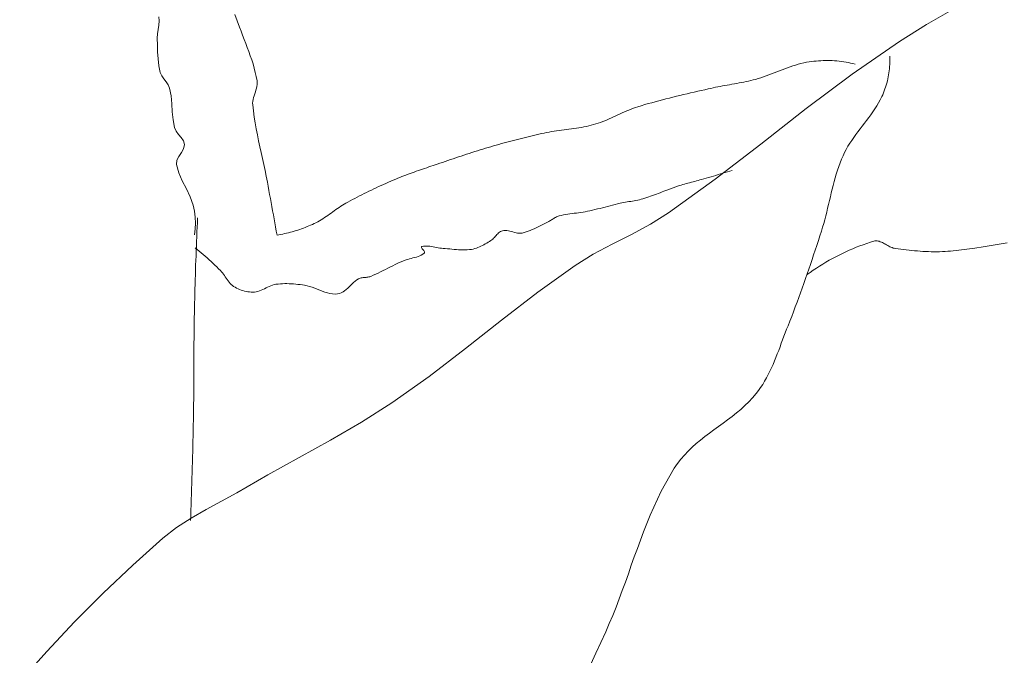
# Model space of a CAD drawing. Units: inches. Extents: x -36302355 to 648, y -221479757 to 75.
# Tile 33 of 37: x 284 to 311, y -20 to -2. Entities that reach past the tile are written whole.
import ezdxf

# ---------------------------------------------------------------- set-up
doc = ezdxf.new("R2010")
doc.units = ezdxf.units.IN
doc.header["$MEASUREMENT"] = 0
doc.layers.add('A-FURN', color=8, linetype='Continuous', lineweight=13)

# ---------------------------------------------------------------- blocks, each defined once
blk = doc.blocks.new('BED-DOUBLE')
for p, q in [((4.128, 63.666), (4.119, 63.783)), ((6.296, 63.67), (6.229, 63.842)), ((26.225, 64.013), (25.45, 63.569)), ((4.097, 63.43), (4.117, 63.548)), ((4.117, 63.548), (4.128, 63.666)), ((6.36, 63.496), (6.296, 63.67)), ((6.401, 63.383), (6.36, 63.496)), ((25.45, 63.569), (24.695, 63.097)), ((4.072, 63.192), (4.078, 63.311)), ((4.078, 63.311), (4.097, 63.43)), ((6.444, 63.269), (6.401, 63.383)), ((6.488, 63.156), (6.444, 63.269)), ((4.076, 62.999), (4.072, 63.192)), ((4.083, 62.806), (4.076, 62.999)), ((6.531, 63.043), (6.488, 63.156)), ((6.574, 62.929), (6.531, 63.043)), ((6.616, 62.816), (6.574, 62.929)), ((24.695, 63.097), (23.379, 62.192)), ((4.096, 62.613), (4.083, 62.806)), ((6.657, 62.702), (6.616, 62.816)), ((6.696, 62.587), (6.657, 62.702)), ((24.428, 62.63), (24.425, 62.688)), ((4.119, 62.421), (4.096, 62.613)), ((4.157, 62.233), (4.119, 62.421)), ((6.733, 62.472), (6.696, 62.587)), ((6.767, 62.356), (6.733, 62.472)), ((21.659, 62.392), (21.585, 62.366)), ((21.733, 62.418), (21.659, 62.392)), ((21.808, 62.442), (21.733, 62.418)), ((21.883, 62.464), (21.808, 62.442)), ((21.958, 62.485), (21.883, 62.464)), ((22.034, 62.503), (21.958, 62.485)), ((22.111, 62.519), (22.034, 62.503)), ((22.188, 62.532), (22.111, 62.519)), ((22.251, 62.541), (22.188, 62.532)), ((22.315, 62.549), (22.251, 62.541)), ((22.378, 62.555), (22.315, 62.549)), ((22.442, 62.561), (22.378, 62.555)), ((22.506, 62.564), (22.442, 62.561)), ((22.57, 62.567), (22.506, 62.564)), ((22.635, 62.568), (22.57, 62.567)), ((22.699, 62.568), (22.635, 62.568)), ((22.763, 62.567), (22.699, 62.568)), ((22.828, 62.565), (22.763, 62.567)), ((22.892, 62.561), (22.828, 62.565)), ((22.956, 62.556), (22.892, 62.561)), ((23.02, 62.55), (22.956, 62.556)), ((23.084, 62.542), (23.02, 62.55)), ((23.148, 62.533), (23.084, 62.542)), ((23.211, 62.523), (23.148, 62.533)), ((23.274, 62.512), (23.211, 62.523)), ((23.337, 62.499), (23.274, 62.512)), ((23.399, 62.485), (23.337, 62.499)), ((23.461, 62.47), (23.399, 62.485)), ((24.417, 62.342), (24.422, 62.4)), ((24.422, 62.4), (24.425, 62.458)), ((24.425, 62.458), (24.428, 62.515)), ((24.428, 62.573), (24.428, 62.63)), ((24.428, 62.515), (24.428, 62.573)), ((4.195, 62.142), (4.157, 62.233)), ((4.253, 62.059), (4.195, 62.142)), ((6.797, 62.24), (6.767, 62.356)), ((6.824, 62.122), (6.797, 62.24)), ((6.846, 62.004), (6.824, 62.122)), ((20.921, 62.115), (20.846, 62.09)), ((20.995, 62.141), (20.921, 62.115)), ((21.069, 62.168), (20.995, 62.141)), ((21.143, 62.196), (21.069, 62.168)), ((21.217, 62.224), (21.143, 62.196)), ((21.29, 62.253), (21.217, 62.224)), ((21.364, 62.282), (21.29, 62.253)), ((21.437, 62.31), (21.364, 62.282)), ((21.511, 62.338), (21.437, 62.31)), ((21.585, 62.366), (21.511, 62.338)), ((23.379, 62.192), (22.102, 61.232)), ((24.371, 62.056), (24.383, 62.113)), ((24.383, 62.113), (24.394, 62.17)), ((24.394, 62.17), (24.403, 62.227)), ((24.403, 62.227), (24.41, 62.285)), ((24.41, 62.285), (24.417, 62.342)), ((4.318, 61.979), (4.253, 62.059)), ((4.377, 61.896), (4.318, 61.979)), ((4.416, 61.805), (4.377, 61.896)), ((6.83, 61.798), (6.842, 61.849)), ((6.842, 61.849), (6.849, 61.9)), ((6.851, 61.952), (6.846, 62.004)), ((6.849, 61.9), (6.851, 61.952)), ((19.645, 61.837), (19.58, 61.824)), ((19.711, 61.849), (19.645, 61.837)), ((19.777, 61.862), (19.711, 61.849)), ((19.843, 61.873), (19.777, 61.862)), ((19.909, 61.885), (19.843, 61.873)), ((19.975, 61.897), (19.909, 61.885)), ((20.041, 61.909), (19.975, 61.897)), ((20.107, 61.92), (20.041, 61.909)), ((20.172, 61.932), (20.107, 61.92)), ((20.238, 61.945), (20.172, 61.932)), ((20.304, 61.957), (20.238, 61.945)), ((20.37, 61.97), (20.304, 61.957)), ((20.435, 61.984), (20.37, 61.97)), ((20.5, 61.998), (20.435, 61.984)), ((20.566, 62.013), (20.5, 61.998)), ((20.631, 62.029), (20.566, 62.013)), ((20.695, 62.046), (20.631, 62.029)), ((20.771, 62.067), (20.695, 62.046)), ((20.846, 62.09), (20.771, 62.067)), ((24.292, 61.778), (24.31, 61.833)), ((24.31, 61.833), (24.327, 61.888)), ((24.327, 61.888), (24.343, 61.944)), ((24.343, 61.944), (24.358, 62)), ((24.358, 62), (24.371, 62.056)), ((4.456, 61.588), (4.416, 61.805)), ((4.476, 61.367), (4.456, 61.588)), ((6.748, 61.541), (6.764, 61.592)), ((6.764, 61.592), (6.781, 61.644)), ((6.781, 61.644), (6.799, 61.695)), ((6.799, 61.695), (6.815, 61.746)), ((6.815, 61.746), (6.83, 61.798)), ((18.498, 61.574), (18.4, 61.551)), ((18.596, 61.598), (18.498, 61.574)), ((18.695, 61.621), (18.596, 61.598)), ((18.793, 61.645), (18.695, 61.621)), ((18.891, 61.667), (18.793, 61.645)), ((18.99, 61.69), (18.891, 61.667)), ((19.088, 61.713), (18.99, 61.69)), ((19.187, 61.736), (19.088, 61.713)), ((19.285, 61.759), (19.187, 61.736)), ((19.383, 61.781), (19.285, 61.759)), ((19.449, 61.796), (19.383, 61.781)), ((19.514, 61.81), (19.449, 61.796)), ((19.58, 61.824), (19.514, 61.81)), ((24.161, 61.478), (24.205, 61.565)), ((24.205, 61.565), (24.228, 61.618)), ((24.228, 61.618), (24.251, 61.67)), ((24.251, 61.67), (24.272, 61.724)), ((24.272, 61.724), (24.292, 61.778)), ((4.49, 61.145), (4.476, 61.367)), ((6.721, 61.386), (6.725, 61.438)), ((6.723, 61.334), (6.721, 61.386)), ((6.742, 61.167), (6.723, 61.334)), ((6.725, 61.438), (6.735, 61.489)), ((6.735, 61.489), (6.748, 61.541)), ((17.426, 61.284), (17.363, 61.264)), ((17.522, 61.314), (17.426, 61.284)), ((17.619, 61.343), (17.522, 61.314)), ((17.716, 61.371), (17.619, 61.343)), ((17.813, 61.398), (17.716, 61.371)), ((17.911, 61.425), (17.813, 61.398)), ((18.008, 61.451), (17.911, 61.425)), ((18.106, 61.477), (18.008, 61.451)), ((18.204, 61.502), (18.106, 61.477)), ((18.302, 61.526), (18.204, 61.502)), ((18.4, 61.551), (18.302, 61.526)), ((24.012, 61.225), (24.064, 61.308)), ((24.064, 61.308), (24.114, 61.392)), ((24.114, 61.392), (24.161, 61.478)), ((4.51, 60.924), (4.49, 61.145)), ((6.765, 61), (6.742, 61.167)), ((16.813, 61.032), (16.752, 61.004)), ((16.873, 61.06), (16.813, 61.032)), ((16.934, 61.087), (16.873, 61.06)), ((16.994, 61.115), (16.934, 61.087)), ((17.055, 61.142), (16.994, 61.115)), ((17.116, 61.168), (17.055, 61.142)), ((17.177, 61.194), (17.116, 61.168)), ((17.238, 61.218), (17.177, 61.194)), ((17.3, 61.242), (17.238, 61.218)), ((17.363, 61.264), (17.3, 61.242)), ((22.102, 61.232), (20.841, 60.248)), ((23.842, 60.984), (23.9, 61.063)), ((23.9, 61.063), (23.957, 61.144)), ((23.957, 61.144), (24.012, 61.225)), ((4.551, 60.707), (4.51, 60.924)), ((6.792, 60.835), (6.765, 61)), ((6.821, 60.669), (6.792, 60.835)), ((15.994, 60.739), (15.926, 60.726)), ((16.062, 60.754), (15.994, 60.739)), ((16.13, 60.771), (16.062, 60.754)), ((16.197, 60.789), (16.13, 60.771)), ((16.261, 60.808), (16.197, 60.789)), ((16.323, 60.828), (16.261, 60.808)), ((16.386, 60.85), (16.323, 60.828)), ((16.448, 60.874), (16.386, 60.85)), ((16.509, 60.898), (16.448, 60.874)), ((16.57, 60.924), (16.509, 60.898)), ((16.631, 60.95), (16.57, 60.924)), ((16.692, 60.977), (16.631, 60.95)), ((16.752, 61.004), (16.692, 60.977)), ((23.602, 60.669), (23.662, 60.748)), ((23.662, 60.748), (23.723, 60.826)), ((23.723, 60.826), (23.783, 60.905)), ((23.783, 60.905), (23.842, 60.984)), ((4.596, 60.607), (4.551, 60.707)), ((4.665, 60.516), (4.596, 60.607)), ((4.738, 60.428), (4.665, 60.516)), ((6.853, 60.504), (6.821, 60.669)), ((6.887, 60.34), (6.853, 60.504)), ((14.45, 60.47), (14.376, 60.452)), ((14.524, 60.487), (14.45, 60.47)), ((14.599, 60.504), (14.524, 60.487)), ((14.673, 60.521), (14.599, 60.504)), ((14.748, 60.538), (14.673, 60.521)), ((14.822, 60.554), (14.748, 60.538)), ((14.891, 60.568), (14.822, 60.554)), ((14.959, 60.581), (14.891, 60.568)), ((15.028, 60.593), (14.959, 60.581)), ((15.097, 60.604), (15.028, 60.593)), ((15.166, 60.614), (15.097, 60.604)), ((15.235, 60.624), (15.166, 60.614)), ((15.304, 60.633), (15.235, 60.624)), ((15.374, 60.642), (15.304, 60.633)), ((15.443, 60.652), (15.374, 60.642)), ((15.512, 60.661), (15.443, 60.652)), ((15.582, 60.67), (15.512, 60.661)), ((15.651, 60.68), (15.582, 60.67)), ((15.72, 60.69), (15.651, 60.68)), ((15.789, 60.701), (15.72, 60.69)), ((15.857, 60.713), (15.789, 60.701)), ((15.926, 60.726), (15.857, 60.713)), ((23.426, 60.431), (23.484, 60.511)), ((23.484, 60.511), (23.542, 60.59)), ((23.542, 60.59), (23.602, 60.669)), ((4.798, 60.335), (4.738, 60.428)), ((4.826, 60.233), (4.798, 60.335)), ((4.805, 60.119), (4.826, 60.233)), ((6.922, 60.175), (6.887, 60.34)), ((13.416, 60.198), (13.343, 60.176)), ((13.489, 60.219), (13.416, 60.198)), ((13.563, 60.239), (13.489, 60.219)), ((13.636, 60.26), (13.563, 60.239)), ((13.71, 60.28), (13.636, 60.26)), ((13.784, 60.3), (13.71, 60.28)), ((13.857, 60.32), (13.784, 60.3)), ((13.931, 60.34), (13.857, 60.32)), ((14.005, 60.359), (13.931, 60.34)), ((14.079, 60.378), (14.005, 60.359)), ((14.153, 60.397), (14.079, 60.378)), ((14.227, 60.416), (14.153, 60.397)), ((14.301, 60.434), (14.227, 60.416)), ((14.376, 60.452), (14.301, 60.434)), ((20.841, 60.248), (19.575, 59.272)), ((23.264, 60.186), (23.316, 60.269)), ((23.316, 60.269), (23.37, 60.351)), ((23.37, 60.351), (23.426, 60.431)), ((4.675, 59.905), (4.746, 60.011)), ((4.746, 60.011), (4.805, 60.119)), ((6.958, 60.011), (6.922, 60.175)), ((6.994, 59.846), (6.958, 60.011)), ((12.519, 59.917), (12.445, 59.892)), ((12.594, 59.942), (12.519, 59.917)), ((12.668, 59.967), (12.594, 59.942)), ((12.743, 59.991), (12.668, 59.967)), ((12.817, 60.015), (12.743, 59.991)), ((12.892, 60.039), (12.817, 60.015)), ((12.967, 60.063), (12.892, 60.039)), ((13.042, 60.086), (12.967, 60.063)), ((13.117, 60.109), (13.042, 60.086)), ((13.192, 60.132), (13.117, 60.109)), ((13.267, 60.154), (13.192, 60.132)), ((13.343, 60.176), (13.267, 60.154)), ((23.085, 59.826), (23.128, 59.926)), ((23.128, 59.926), (23.17, 60.015)), ((23.17, 60.015), (23.215, 60.101)), ((23.215, 60.101), (23.264, 60.186)), ((4.607, 59.685), (4.62, 59.798)), ((4.668, 59.449), (4.607, 59.685)), ((4.62, 59.798), (4.675, 59.905)), ((7.03, 59.682), (6.994, 59.846)), ((7.066, 59.517), (7.03, 59.682)), ((11.734, 59.651), (11.676, 59.631)), ((11.792, 59.671), (11.734, 59.651)), ((11.85, 59.69), (11.792, 59.671)), ((11.924, 59.716), (11.85, 59.69)), ((11.999, 59.741), (11.924, 59.716)), ((12.073, 59.766), (11.999, 59.741)), ((12.147, 59.792), (12.073, 59.766)), ((12.221, 59.817), (12.147, 59.792)), ((12.296, 59.842), (12.221, 59.817)), ((12.37, 59.867), (12.296, 59.842)), ((12.445, 59.892), (12.37, 59.867)), ((23.007, 59.623), (23.045, 59.725)), ((23.045, 59.725), (23.085, 59.826)), ((4.766, 59.224), (4.668, 59.449)), ((7.1, 59.353), (7.066, 59.517)), ((10.924, 59.366), (10.867, 59.344)), ((10.981, 59.388), (10.924, 59.366)), ((11.039, 59.41), (10.981, 59.388)), ((11.096, 59.431), (11.039, 59.41)), ((11.154, 59.452), (11.096, 59.431)), ((11.212, 59.472), (11.154, 59.452)), ((11.269, 59.493), (11.212, 59.472)), ((11.327, 59.513), (11.269, 59.493)), ((11.385, 59.533), (11.327, 59.513)), ((11.443, 59.553), (11.385, 59.533)), ((11.501, 59.572), (11.443, 59.553)), ((11.56, 59.592), (11.501, 59.572)), ((11.618, 59.612), (11.56, 59.592)), ((11.676, 59.631), (11.618, 59.612)), ((19.588, 59.379), (19.523, 59.36)), ((19.653, 59.399), (19.588, 59.379)), ((19.718, 59.418), (19.653, 59.399)), ((19.783, 59.438), (19.718, 59.418)), ((19.848, 59.458), (19.783, 59.438)), ((19.913, 59.478), (19.848, 59.458)), ((19.978, 59.498), (19.913, 59.478)), ((20.043, 59.518), (19.978, 59.498)), ((22.909, 59.313), (22.94, 59.417)), ((22.94, 59.417), (22.973, 59.521)), ((22.973, 59.521), (23.007, 59.623)), ((4.88, 59.003), (4.766, 59.224)), ((7.132, 59.188), (7.1, 59.353)), ((7.153, 59.075), (7.132, 59.188)), ((10.29, 59.097), (10.223, 59.066)), ((10.358, 59.127), (10.29, 59.097)), ((10.425, 59.157), (10.358, 59.127)), ((10.493, 59.187), (10.425, 59.157)), ((10.561, 59.216), (10.493, 59.187)), ((10.629, 59.246), (10.561, 59.216)), ((10.697, 59.275), (10.629, 59.246)), ((10.753, 59.298), (10.697, 59.275)), ((10.81, 59.321), (10.753, 59.298)), ((10.867, 59.344), (10.81, 59.321)), ((19.575, 59.272), (18.281, 58.335)), ((18.58, 59.094), (18.555, 59.086)), ((18.627, 59.108), (18.58, 59.094)), ((18.675, 59.122), (18.627, 59.108)), ((18.722, 59.135), (18.675, 59.122)), ((18.769, 59.149), (18.722, 59.135)), ((18.817, 59.161), (18.769, 59.149)), ((18.864, 59.174), (18.817, 59.161)), ((18.912, 59.187), (18.864, 59.174)), ((18.959, 59.199), (18.912, 59.187)), ((19.007, 59.212), (18.959, 59.199)), ((19.054, 59.225), (19.007, 59.212)), ((19.102, 59.238), (19.054, 59.225)), ((19.149, 59.251), (19.102, 59.238)), ((19.197, 59.264), (19.149, 59.251)), ((19.262, 59.283), (19.197, 59.264)), ((19.327, 59.302), (19.262, 59.283)), ((19.392, 59.321), (19.327, 59.302)), ((19.458, 59.341), (19.392, 59.321)), ((19.523, 59.36), (19.458, 59.341)), ((22.826, 58.996), (22.852, 59.102)), ((22.852, 59.102), (22.88, 59.208)), ((22.88, 59.208), (22.909, 59.313)), ((4.988, 58.78), (4.88, 59.003)), ((7.174, 58.962), (7.153, 59.075)), ((7.195, 58.849), (7.174, 58.962)), ((7.216, 58.737), (7.195, 58.849)), ((9.756, 58.842), (9.69, 58.809)), ((9.822, 58.875), (9.756, 58.842)), ((9.889, 58.908), (9.822, 58.875)), ((9.955, 58.94), (9.889, 58.908)), ((10.022, 58.972), (9.955, 58.94)), ((10.089, 59.004), (10.022, 58.972)), ((10.156, 59.035), (10.089, 59.004)), ((10.223, 59.066), (10.156, 59.035)), ((17.887, 58.837), (17.834, 58.817)), ((17.94, 58.857), (17.887, 58.837)), ((17.993, 58.877), (17.94, 58.857)), ((18.046, 58.898), (17.993, 58.877)), ((18.098, 58.918), (18.046, 58.898)), ((18.151, 58.938), (18.098, 58.918)), ((18.204, 58.958), (18.151, 58.938)), ((18.257, 58.978), (18.204, 58.958)), ((18.282, 58.987), (18.257, 58.978)), ((18.307, 58.996), (18.282, 58.987)), ((18.332, 59.005), (18.307, 58.996)), ((18.356, 59.015), (18.332, 59.005)), ((18.381, 59.024), (18.356, 59.015)), ((18.406, 59.033), (18.381, 59.024)), ((18.431, 59.043), (18.406, 59.033)), ((18.455, 59.052), (18.431, 59.043)), ((18.48, 59.061), (18.455, 59.052)), ((18.505, 59.07), (18.48, 59.061)), ((18.53, 59.078), (18.505, 59.07)), ((18.555, 59.086), (18.53, 59.078)), ((22.775, 58.784), (22.8, 58.89)), ((22.8, 58.89), (22.826, 58.996)), ((5.069, 58.548), (4.988, 58.78)), ((5.103, 58.387), (5.069, 58.548)), ((7.236, 58.624), (7.216, 58.737)), ((7.257, 58.511), (7.236, 58.624)), ((9.22, 58.553), (9.174, 58.522)), ((9.267, 58.582), (9.22, 58.553)), ((9.315, 58.61), (9.267, 58.582)), ((9.363, 58.637), (9.315, 58.61)), ((9.428, 58.672), (9.363, 58.637)), ((9.493, 58.707), (9.428, 58.672)), ((9.559, 58.741), (9.493, 58.707)), ((9.624, 58.776), (9.559, 58.741)), ((9.69, 58.809), (9.624, 58.776)), ((16.723, 58.554), (16.653, 58.536)), ((16.792, 58.571), (16.723, 58.554)), ((16.862, 58.588), (16.792, 58.571)), ((16.933, 58.604), (16.862, 58.588)), ((16.981, 58.615), (16.933, 58.604)), ((17.03, 58.624), (16.981, 58.615)), ((17.079, 58.633), (17.03, 58.624)), ((17.128, 58.642), (17.079, 58.633)), ((17.177, 58.65), (17.128, 58.642)), ((17.226, 58.658), (17.177, 58.65)), ((17.275, 58.666), (17.226, 58.658)), ((17.324, 58.675), (17.275, 58.666)), ((17.372, 58.684), (17.324, 58.675)), ((17.421, 58.693), (17.372, 58.684)), ((17.469, 58.704), (17.421, 58.693)), ((17.518, 58.716), (17.469, 58.704)), ((17.566, 58.728), (17.518, 58.716)), ((17.62, 58.744), (17.566, 58.728)), ((17.674, 58.761), (17.62, 58.744)), ((17.727, 58.779), (17.674, 58.761)), ((17.781, 58.798), (17.727, 58.779)), ((17.834, 58.817), (17.781, 58.798)), ((22.699, 58.465), (22.725, 58.571)), ((22.725, 58.571), (22.75, 58.678)), ((22.75, 58.678), (22.775, 58.784)), ((5.123, 58.222), (5.103, 58.387)), ((7.278, 58.398), (7.257, 58.511)), ((7.298, 58.285), (7.278, 58.398)), ((7.319, 58.172), (7.298, 58.285)), ((8.856, 58.299), (8.81, 58.267)), ((8.901, 58.331), (8.856, 58.299)), ((8.946, 58.364), (8.901, 58.331)), ((8.991, 58.396), (8.946, 58.364)), ((9.037, 58.428), (8.991, 58.396)), ((9.082, 58.46), (9.037, 58.428)), ((9.128, 58.491), (9.082, 58.46)), ((9.174, 58.522), (9.128, 58.491)), ((15.355, 58.28), (15.295, 58.267)), ((15.415, 58.291), (15.355, 58.28)), ((15.476, 58.301), (15.415, 58.291)), ((15.536, 58.31), (15.476, 58.301)), ((15.597, 58.318), (15.536, 58.31)), ((15.658, 58.326), (15.597, 58.318)), ((15.719, 58.333), (15.658, 58.326)), ((15.78, 58.341), (15.719, 58.333)), ((15.841, 58.35), (15.78, 58.341)), ((15.902, 58.359), (15.841, 58.35)), ((15.963, 58.369), (15.902, 58.359)), ((16.023, 58.381), (15.963, 58.369)), ((16.093, 58.396), (16.023, 58.381)), ((16.164, 58.412), (16.093, 58.396)), ((16.234, 58.428), (16.164, 58.412)), ((16.304, 58.446), (16.234, 58.428)), ((16.374, 58.463), (16.304, 58.446)), ((16.443, 58.481), (16.374, 58.463)), ((16.513, 58.5), (16.443, 58.481)), ((16.583, 58.518), (16.513, 58.5)), ((16.653, 58.536), (16.583, 58.518)), ((18.281, 58.335), (17.775, 58.02)), ((22.647, 58.252), (22.674, 58.358)), ((22.674, 58.358), (22.699, 58.465)), ((5.13, 58.056), (5.123, 58.222)), ((5.124, 57.891), (5.13, 58.056)), ((5.181, 57.938), (5.187, 58.07)), ((5.187, 58.07), (5.194, 58.202)), ((7.339, 58.06), (7.319, 58.172)), ((7.36, 57.947), (7.339, 58.06)), ((8.382, 58.018), (8.333, 57.996)), ((8.431, 58.041), (8.382, 58.018)), ((8.481, 58.065), (8.431, 58.041)), ((8.53, 58.09), (8.481, 58.065)), ((8.578, 58.117), (8.53, 58.09)), ((8.626, 58.146), (8.578, 58.117)), ((8.672, 58.175), (8.626, 58.146)), ((8.719, 58.205), (8.672, 58.175)), ((8.765, 58.236), (8.719, 58.205)), ((8.81, 58.267), (8.765, 58.236)), ((14.766, 58.009), (14.711, 57.981)), ((14.82, 58.037), (14.766, 58.009)), ((14.874, 58.064), (14.82, 58.037)), ((14.929, 58.09), (14.874, 58.064)), ((14.953, 58.102), (14.929, 58.09)), ((14.976, 58.115), (14.953, 58.102)), ((15, 58.128), (14.976, 58.115)), ((15.022, 58.143), (15, 58.128)), ((15.045, 58.157), (15.022, 58.143)), ((15.068, 58.171), (15.045, 58.157)), ((15.091, 58.186), (15.068, 58.171)), ((15.114, 58.199), (15.091, 58.186)), ((15.137, 58.213), (15.114, 58.199)), ((15.161, 58.225), (15.137, 58.213)), ((15.185, 58.236), (15.161, 58.225)), ((15.21, 58.245), (15.185, 58.236)), ((15.235, 58.253), (15.21, 58.245)), ((15.295, 58.267), (15.235, 58.253)), ((17.775, 58.02), (17.248, 57.739)), ((22.56, 57.937), (22.59, 58.042)), ((22.59, 58.042), (22.619, 58.147)), ((22.619, 58.147), (22.647, 58.252)), ((5.104, 57.727), (5.124, 57.891)), ((5.17, 57.675), (5.176, 57.807)), ((5.176, 57.807), (5.181, 57.938)), ((7.38, 57.834), (7.36, 57.947)), ((7.4, 57.721), (7.38, 57.834)), ((7.453, 57.73), (7.4, 57.721)), ((7.506, 57.74), (7.453, 57.73)), ((7.559, 57.751), (7.506, 57.74)), ((7.612, 57.762), (7.559, 57.751)), ((7.665, 57.774), (7.612, 57.762)), ((7.718, 57.787), (7.665, 57.774)), ((7.77, 57.801), (7.718, 57.787)), ((7.823, 57.815), (7.77, 57.801)), ((7.875, 57.83), (7.823, 57.815)), ((7.927, 57.846), (7.875, 57.83)), ((7.978, 57.862), (7.927, 57.846)), ((8.03, 57.879), (7.978, 57.862)), ((8.081, 57.897), (8.03, 57.879)), ((8.132, 57.916), (8.081, 57.897)), ((8.183, 57.935), (8.132, 57.916)), ((8.233, 57.955), (8.183, 57.935)), ((8.283, 57.975), (8.233, 57.955)), ((8.333, 57.996), (8.283, 57.975)), ((13.509, 57.734), (13.486, 57.709)), ((13.531, 57.758), (13.509, 57.734)), ((13.554, 57.781), (13.531, 57.758)), ((13.579, 57.801), (13.554, 57.781)), ((13.605, 57.819), (13.579, 57.801)), ((13.633, 57.832), (13.605, 57.819)), ((13.663, 57.842), (13.633, 57.832)), ((13.704, 57.849), (13.663, 57.842)), ((13.746, 57.85), (13.704, 57.849)), ((13.787, 57.847), (13.746, 57.85)), ((13.829, 57.84), (13.787, 57.847)), ((13.871, 57.83), (13.829, 57.84)), ((13.914, 57.819), (13.871, 57.83)), ((13.956, 57.807), (13.914, 57.819)), ((13.998, 57.795), (13.956, 57.807)), ((14.04, 57.785), (13.998, 57.795)), ((14.082, 57.778), (14.04, 57.785)), ((14.124, 57.773), (14.082, 57.778)), ((14.166, 57.773), (14.124, 57.773)), ((14.208, 57.778), (14.166, 57.773)), ((14.266, 57.791), (14.208, 57.778)), ((14.324, 57.808), (14.266, 57.791)), ((14.381, 57.827), (14.324, 57.808)), ((14.437, 57.849), (14.381, 57.827)), ((14.493, 57.873), (14.437, 57.849)), ((14.548, 57.899), (14.493, 57.873)), ((14.603, 57.925), (14.548, 57.899)), ((14.657, 57.953), (14.603, 57.925)), ((14.711, 57.981), (14.657, 57.953)), ((17.248, 57.739), (16.714, 57.469)), ((22.484, 57.701), (22.527, 57.833)), ((22.527, 57.833), (22.56, 57.937)), ((5.159, 57.411), (5.164, 57.543)), ((5.164, 57.543), (5.17, 57.675)), ((13.146, 57.454), (13.106, 57.432)), ((13.186, 57.477), (13.146, 57.454)), ((13.226, 57.5), (13.186, 57.477)), ((13.266, 57.523), (13.226, 57.5)), ((13.305, 57.547), (13.266, 57.523)), ((13.344, 57.571), (13.305, 57.547)), ((13.371, 57.589), (13.344, 57.571)), ((13.396, 57.61), (13.371, 57.589)), ((13.419, 57.633), (13.396, 57.61)), ((13.442, 57.658), (13.419, 57.633)), ((13.464, 57.683), (13.442, 57.658)), ((13.486, 57.709), (13.464, 57.683)), ((16.714, 57.469), (16.186, 57.189)), ((22.398, 57.436), (22.441, 57.568)), ((22.441, 57.568), (22.484, 57.701)), ((23.688, 57.454), (23.59, 57.418)), ((23.786, 57.488), (23.688, 57.454)), ((23.885, 57.52), (23.786, 57.488)), ((23.984, 57.551), (23.885, 57.52)), ((24.014, 57.558), (23.984, 57.551)), ((24.044, 57.56), (24.014, 57.558)), ((24.074, 57.559), (24.044, 57.56)), ((24.103, 57.555), (24.074, 57.559)), ((24.133, 57.548), (24.103, 57.555)), ((24.162, 57.538), (24.133, 57.548)), ((24.191, 57.526), (24.162, 57.538)), ((24.22, 57.513), (24.191, 57.526)), ((24.25, 57.498), (24.22, 57.513)), ((24.279, 57.482), (24.25, 57.498)), ((24.308, 57.465), (24.279, 57.482)), ((24.338, 57.448), (24.308, 57.465)), ((27.467, 57.465), (27.243, 57.428)), ((27.691, 57.503), (27.467, 57.465)), ((5.185, 57.325), (5.129, 57.371)), ((5.149, 57.147), (5.154, 57.279)), ((5.154, 57.279), (5.159, 57.411)), ((5.24, 57.278), (5.185, 57.325)), ((5.295, 57.231), (5.24, 57.278)), ((5.35, 57.183), (5.295, 57.231)), ((5.405, 57.135), (5.35, 57.183)), ((11.451, 57.188), (11.409, 57.165)), ((11.414, 57.394), (11.411, 57.385)), ((11.411, 57.385), (11.414, 57.373)), ((11.425, 57.4), (11.414, 57.394)), ((11.414, 57.373), (11.422, 57.359)), ((11.422, 57.359), (11.433, 57.343)), ((11.469, 57.409), (11.425, 57.4)), ((11.433, 57.343), (11.447, 57.325)), ((11.447, 57.325), (11.461, 57.307)), ((11.491, 57.216), (11.451, 57.188)), ((11.461, 57.307), (11.475, 57.289)), ((11.514, 57.414), (11.469, 57.409)), ((11.475, 57.289), (11.487, 57.271)), ((11.487, 57.271), (11.496, 57.255)), ((11.5, 57.226), (11.491, 57.216)), ((11.496, 57.255), (11.501, 57.239)), ((11.501, 57.239), (11.5, 57.226)), ((11.559, 57.415), (11.514, 57.414)), ((11.604, 57.413), (11.559, 57.415)), ((11.649, 57.409), (11.604, 57.413)), ((11.695, 57.403), (11.649, 57.409)), ((11.741, 57.395), (11.695, 57.403)), ((11.787, 57.386), (11.741, 57.395)), ((11.832, 57.378), (11.787, 57.386)), ((11.878, 57.369), (11.832, 57.378)), ((11.924, 57.362), (11.878, 57.369)), ((11.97, 57.356), (11.924, 57.362)), ((12.015, 57.352), (11.97, 57.356)), ((12.076, 57.348), (12.015, 57.352)), ((12.137, 57.343), (12.076, 57.348)), ((12.198, 57.338), (12.137, 57.343)), ((12.26, 57.331), (12.198, 57.338)), ((12.321, 57.325), (12.26, 57.331)), ((12.382, 57.32), (12.321, 57.325)), ((12.443, 57.315), (12.382, 57.32)), ((12.504, 57.311), (12.443, 57.315)), ((12.565, 57.309), (12.504, 57.311)), ((12.626, 57.309), (12.565, 57.309)), ((12.686, 57.312), (12.626, 57.309)), ((12.747, 57.317), (12.686, 57.312)), ((12.807, 57.325), (12.747, 57.317)), ((12.852, 57.334), (12.807, 57.325)), ((12.895, 57.345), (12.852, 57.334)), ((12.939, 57.359), (12.895, 57.345)), ((12.981, 57.375), (12.939, 57.359)), ((13.023, 57.392), (12.981, 57.375)), ((13.065, 57.412), (13.023, 57.392)), ((13.106, 57.432), (13.065, 57.412)), ((16.186, 57.189), (15.68, 56.875)), ((22.31, 57.171), (22.354, 57.303)), ((22.354, 57.303), (22.398, 57.436)), ((23.11, 57.213), (23.017, 57.167)), ((23.205, 57.258), (23.11, 57.213)), ((23.3, 57.3), (23.205, 57.258)), ((23.396, 57.341), (23.3, 57.3)), ((23.493, 57.381), (23.396, 57.341)), ((23.59, 57.418), (23.493, 57.381)), ((24.367, 57.431), (24.338, 57.448)), ((24.397, 57.415), (24.367, 57.431)), ((24.426, 57.399), (24.397, 57.415)), ((24.456, 57.385), (24.426, 57.399)), ((24.487, 57.372), (24.456, 57.385)), ((24.517, 57.362), (24.487, 57.372)), ((24.548, 57.354), (24.517, 57.362)), ((24.579, 57.348), (24.548, 57.354)), ((24.655, 57.338), (24.579, 57.348)), ((24.732, 57.329), (24.655, 57.338)), ((24.808, 57.32), (24.732, 57.329)), ((24.885, 57.311), (24.808, 57.32)), ((24.962, 57.302), (24.885, 57.311)), ((25.039, 57.294), (24.962, 57.302)), ((25.116, 57.287), (25.039, 57.294)), ((25.193, 57.28), (25.116, 57.287)), ((25.27, 57.274), (25.193, 57.28)), ((25.347, 57.269), (25.27, 57.274)), ((25.424, 57.264), (25.347, 57.269)), ((25.501, 57.261), (25.424, 57.264)), ((25.578, 57.258), (25.501, 57.261)), ((25.655, 57.257), (25.578, 57.258)), ((25.732, 57.257), (25.655, 57.257)), ((25.809, 57.258), (25.732, 57.257)), ((25.886, 57.261), (25.809, 57.258)), ((25.963, 57.265), (25.886, 57.261)), ((26.039, 57.27), (25.963, 57.265)), ((26.116, 57.277), (26.039, 57.27)), ((26.342, 57.302), (26.116, 57.277)), ((26.568, 57.329), (26.342, 57.302)), ((26.793, 57.36), (26.568, 57.329)), ((27.018, 57.393), (26.793, 57.36)), ((27.243, 57.428), (27.018, 57.393)), ((5.139, 56.883), (5.144, 57.015)), ((5.144, 57.015), (5.149, 57.147)), ((5.459, 57.087), (5.405, 57.135)), ((5.513, 57.038), (5.459, 57.087)), ((5.566, 56.989), (5.513, 57.038)), ((5.619, 56.939), (5.566, 56.989)), ((5.671, 56.889), (5.619, 56.939)), ((10.754, 56.937), (10.685, 56.904)), ((10.822, 56.969), (10.754, 56.937)), ((10.892, 56.999), (10.822, 56.969)), ((10.937, 57.017), (10.892, 56.999)), ((10.984, 57.033), (10.937, 57.017)), ((11.032, 57.047), (10.984, 57.033)), ((11.08, 57.06), (11.032, 57.047)), ((11.129, 57.073), (11.08, 57.06)), ((11.177, 57.085), (11.129, 57.073)), ((11.225, 57.098), (11.177, 57.085)), ((11.273, 57.111), (11.225, 57.098)), ((11.319, 57.127), (11.273, 57.111)), ((11.365, 57.144), (11.319, 57.127)), ((11.409, 57.165), (11.365, 57.144)), ((22.177, 56.774), (22.221, 56.906)), ((22.221, 56.906), (22.266, 57.039)), ((22.266, 57.039), (22.31, 57.171)), ((22.561, 56.913), (22.472, 56.858)), ((22.65, 56.967), (22.561, 56.913)), ((22.74, 57.02), (22.65, 56.967)), ((22.831, 57.07), (22.74, 57.02)), ((22.924, 57.12), (22.831, 57.07)), ((23.017, 57.167), (22.924, 57.12)), ((5.131, 56.619), (5.135, 56.751)), ((5.135, 56.751), (5.139, 56.883)), ((5.723, 56.839), (5.671, 56.889)), ((5.775, 56.788), (5.723, 56.839)), ((5.826, 56.736), (5.775, 56.788)), ((5.856, 56.704), (5.826, 56.736)), ((5.885, 56.67), (5.856, 56.704)), ((5.911, 56.634), (5.885, 56.67)), ((5.937, 56.597), (5.911, 56.634)), ((10.142, 56.634), (10.073, 56.604)), ((10.211, 56.666), (10.142, 56.634)), ((10.279, 56.699), (10.211, 56.666)), ((10.347, 56.733), (10.279, 56.699)), ((10.414, 56.767), (10.347, 56.733)), ((10.482, 56.801), (10.414, 56.767)), ((10.55, 56.836), (10.482, 56.801)), ((10.617, 56.87), (10.55, 56.836)), ((10.685, 56.904), (10.617, 56.87)), ((15.68, 56.875), (14.648, 56.132)), ((22.086, 56.511), (22.131, 56.643)), ((22.214, 56.683), (22.13, 56.622)), ((22.131, 56.643), (22.177, 56.774)), ((22.299, 56.743), (22.214, 56.683)), ((22.385, 56.801), (22.299, 56.743)), ((22.472, 56.858), (22.385, 56.801)), ((5.123, 56.355), (5.127, 56.487)), ((5.127, 56.487), (5.131, 56.619)), ((5.962, 56.559), (5.937, 56.597)), ((5.987, 56.522), (5.962, 56.559)), ((6.013, 56.485), (5.987, 56.522)), ((6.039, 56.449), (6.013, 56.485)), ((6.066, 56.414), (6.039, 56.449)), ((6.095, 56.38), (6.066, 56.414)), ((6.125, 56.349), (6.095, 56.38)), ((7.432, 56.362), (7.371, 56.355)), ((7.492, 56.368), (7.432, 56.362)), ((7.553, 56.371), (7.492, 56.368)), ((7.614, 56.373), (7.553, 56.371)), ((7.676, 56.373), (7.614, 56.373)), ((7.737, 56.371), (7.676, 56.373)), ((7.798, 56.369), (7.737, 56.371)), ((7.859, 56.365), (7.798, 56.369)), ((7.92, 56.359), (7.859, 56.365)), ((7.981, 56.353), (7.92, 56.359)), ((9.486, 56.366), (9.445, 56.325)), ((9.528, 56.405), (9.486, 56.366)), ((9.571, 56.442), (9.528, 56.405)), ((9.616, 56.476), (9.571, 56.442)), ((9.663, 56.504), (9.616, 56.476)), ((9.687, 56.515), (9.663, 56.504)), ((9.712, 56.524), (9.687, 56.515)), ((9.738, 56.53), (9.712, 56.524)), ((9.764, 56.535), (9.738, 56.53)), ((9.79, 56.539), (9.764, 56.535)), ((9.817, 56.542), (9.79, 56.539)), ((9.844, 56.545), (9.817, 56.542)), ((9.872, 56.547), (9.844, 56.545)), ((9.899, 56.55), (9.872, 56.547)), ((9.925, 56.554), (9.899, 56.55)), ((9.952, 56.559), (9.925, 56.554)), ((9.977, 56.566), (9.952, 56.559)), ((10.003, 56.574), (9.977, 56.566)), ((10.073, 56.604), (10.003, 56.574)), ((21.993, 56.248), (22.039, 56.379)), ((22.039, 56.379), (22.086, 56.511)), ((5.112, 55.959), (5.115, 56.091)), ((5.115, 56.091), (5.119, 56.223)), ((5.119, 56.223), (5.123, 56.355)), ((6.158, 56.321), (6.125, 56.349)), ((6.194, 56.296), (6.158, 56.321)), ((6.234, 56.272), (6.194, 56.296)), ((6.274, 56.25), (6.234, 56.272)), ((6.317, 56.229), (6.274, 56.25)), ((6.36, 56.211), (6.317, 56.229)), ((6.404, 56.195), (6.36, 56.211)), ((6.449, 56.18), (6.404, 56.195)), ((6.494, 56.168), (6.449, 56.18)), ((6.54, 56.157), (6.494, 56.168)), ((6.586, 56.149), (6.54, 56.157)), ((6.633, 56.143), (6.586, 56.149)), ((6.679, 56.139), (6.633, 56.143)), ((6.725, 56.138), (6.679, 56.139)), ((6.772, 56.139), (6.725, 56.138)), ((6.82, 56.144), (6.772, 56.139)), ((6.867, 56.155), (6.82, 56.144)), ((6.914, 56.169), (6.867, 56.155)), ((6.959, 56.187), (6.914, 56.169)), ((7.005, 56.207), (6.959, 56.187)), ((7.05, 56.229), (7.005, 56.207)), ((7.094, 56.252), (7.05, 56.229)), ((7.139, 56.274), (7.094, 56.252)), ((7.184, 56.296), (7.139, 56.274)), ((7.23, 56.316), (7.184, 56.296)), ((7.276, 56.333), (7.23, 56.316)), ((7.323, 56.346), (7.276, 56.333)), ((7.371, 56.355), (7.323, 56.346)), ((8.042, 56.345), (7.981, 56.353)), ((8.103, 56.337), (8.042, 56.345)), ((8.163, 56.328), (8.103, 56.337)), ((8.235, 56.314), (8.163, 56.328)), ((8.306, 56.294), (8.235, 56.314)), ((8.377, 56.271), (8.306, 56.294)), ((8.448, 56.244), (8.377, 56.271)), ((8.518, 56.217), (8.448, 56.244)), ((8.588, 56.189), (8.518, 56.217)), ((8.658, 56.162), (8.588, 56.189)), ((8.728, 56.137), (8.658, 56.162)), ((8.798, 56.115), (8.728, 56.137)), ((8.869, 56.098), (8.798, 56.115)), ((8.94, 56.087), (8.869, 56.098)), ((9.011, 56.083), (8.94, 56.087)), ((9.084, 56.087), (9.011, 56.083)), ((9.137, 56.097), (9.084, 56.087)), ((9.186, 56.116), (9.137, 56.097)), ((9.233, 56.141), (9.186, 56.116)), ((9.278, 56.171), (9.233, 56.141)), ((9.321, 56.206), (9.278, 56.171)), ((9.363, 56.244), (9.321, 56.206)), ((9.404, 56.284), (9.363, 56.244)), ((9.445, 56.325), (9.404, 56.284)), ((14.648, 56.132), (13.641, 55.355)), ((21.898, 55.986), (21.946, 56.117)), ((21.946, 56.117), (21.993, 56.248)), ((5.106, 55.695), (5.109, 55.827)), ((5.109, 55.827), (5.112, 55.959)), ((21.801, 55.724), (21.85, 55.855)), ((21.85, 55.855), (21.898, 55.986)), ((5.1, 55.422), (5.103, 55.563)), ((5.103, 55.563), (5.106, 55.695)), ((21.701, 55.464), (21.751, 55.594)), ((21.751, 55.594), (21.801, 55.724)), ((5.096, 55.14), (5.098, 55.281)), ((5.098, 55.281), (5.1, 55.422)), ((13.641, 55.355), (12.64, 54.568)), ((21.599, 55.205), (21.65, 55.334)), ((21.65, 55.334), (21.701, 55.464)), ((5.093, 54.857), (5.094, 54.999)), ((5.094, 54.999), (5.096, 55.14)), ((21.486, 54.912), (21.523, 55.01)), ((21.523, 55.01), (21.56, 55.108)), ((21.56, 55.108), (21.599, 55.205)), ((5.091, 54.575), (5.092, 54.716)), ((5.092, 54.716), (5.093, 54.857)), ((21.375, 54.617), (21.412, 54.715)), ((21.412, 54.715), (21.449, 54.814)), ((21.449, 54.814), (21.486, 54.912)), ((5.091, 54.434), (5.091, 54.575)), ((12.64, 54.568), (11.629, 53.795)), ((21.3, 54.42), (21.338, 54.518)), ((21.338, 54.518), (21.375, 54.617)), ((5.09, 54.293), (5.091, 54.434)), ((5.09, 54.152), (5.09, 54.293)), ((21.181, 54.129), (21.222, 54.225)), ((21.222, 54.225), (21.261, 54.323)), ((21.261, 54.323), (21.3, 54.42)), ((5.089, 54.01), (5.09, 54.152)), ((5.089, 53.869), (5.089, 54.01)), ((21.047, 53.846), (21.093, 53.939)), ((21.093, 53.939), (21.138, 54.034)), ((21.138, 54.034), (21.181, 54.129)), ((5.088, 53.728), (5.089, 53.869)), ((5.088, 53.587), (5.088, 53.728)), ((11.629, 53.795), (10.592, 53.06)), ((20.894, 53.576), (20.947, 53.664)), ((20.947, 53.664), (20.998, 53.754)), ((20.998, 53.754), (21.047, 53.846)), ((5.086, 53.304), (5.087, 53.446)), ((5.087, 53.446), (5.088, 53.587)), ((20.714, 53.322), (20.777, 53.405)), ((20.777, 53.405), (20.837, 53.489)), ((20.837, 53.489), (20.894, 53.576)), ((5.083, 53.022), (5.085, 53.163)), ((5.085, 53.163), (5.086, 53.304)), ((20.399, 52.986), (20.509, 53.093)), ((20.509, 53.093), (20.615, 53.205)), ((20.615, 53.205), (20.714, 53.322)), ((5.078, 52.74), (5.081, 52.881)), ((5.081, 52.881), (5.083, 53.022)), ((10.592, 53.06), (9.751, 52.527)), ((20.165, 52.782), (20.284, 52.882)), ((20.284, 52.882), (20.399, 52.986)), ((5.073, 52.445), (5.076, 52.592)), ((5.076, 52.592), (5.078, 52.74)), ((19.794, 52.496), (19.919, 52.59)), ((19.919, 52.59), (20.043, 52.685)), ((20.043, 52.685), (20.165, 52.782)), ((5.066, 52.15), (5.07, 52.297)), ((5.07, 52.297), (5.073, 52.445)), ((9.751, 52.527), (8.89, 52.026)), ((19.416, 52.218), (19.541, 52.311)), ((19.541, 52.311), (19.668, 52.404)), ((19.668, 52.404), (19.794, 52.496)), ((5.059, 51.855), (5.063, 52.002)), ((5.063, 52.002), (5.066, 52.15)), ((8.89, 52.026), (8.018, 51.542)), ((19.05, 51.929), (19.169, 52.027)), ((19.169, 52.027), (19.291, 52.124)), ((19.291, 52.124), (19.416, 52.218)), ((5.052, 51.56), (5.056, 51.708)), ((5.056, 51.708), (5.059, 51.855)), ((18.718, 51.612), (18.824, 51.722)), ((18.824, 51.722), (18.935, 51.827)), ((18.935, 51.827), (19.05, 51.929)), ((5.048, 51.413), (5.052, 51.56)), ((8.018, 51.542), (7.145, 51.061)), ((18.524, 51.377), (18.617, 51.498)), ((18.617, 51.498), (18.718, 51.612)), ((5.04, 51.118), (5.044, 51.265)), ((5.044, 51.265), (5.048, 51.413)), ((18.31, 51.04), (18.438, 51.25)), ((18.438, 51.25), (18.524, 51.377)), ((5.031, 50.823), (5.035, 50.97)), ((5.035, 50.97), (5.04, 51.118)), ((7.145, 51.061), (6.279, 50.567)), ((18.19, 50.826), (18.31, 51.04)), ((5.021, 50.528), (5.026, 50.675)), ((5.026, 50.675), (5.031, 50.823)), ((18.076, 50.609), (18.19, 50.826)), ((5.011, 50.233), (5.016, 50.381)), ((5.016, 50.381), (5.021, 50.528)), ((6.279, 50.567), (5.859, 50.33)), ((17.866, 50.165), (17.968, 50.388)), ((17.968, 50.388), (18.076, 50.609)), ((5.001, 49.938), (5.006, 50.086)), ((5.006, 50.086), (5.011, 50.233)), ((5.434, 50.099), (5.015, 49.86)), ((5.859, 50.33), (5.434, 50.099)), ((17.768, 49.939), (17.866, 50.165)), ((5.015, 49.86), (4.61, 49.601)), ((4.995, 49.791), (5.001, 49.938)), ((17.674, 49.711), (17.768, 49.939)), ((4.61, 49.601), (4.231, 49.307)), ((17.584, 49.482), (17.674, 49.711)), ((4.231, 49.307), (3.391, 48.555)), ((17.411, 49.018), (17.496, 49.25)), ((17.496, 49.25), (17.584, 49.482)), ((17.327, 48.785), (17.411, 49.018)), ((17.244, 48.552), (17.327, 48.785)), ((3.391, 48.555), (2.572, 47.778)), ((17.161, 48.318), (17.244, 48.552)), ((17.078, 48.085), (17.161, 48.318)), ((16.994, 47.852), (17.078, 48.085)), ((2.572, 47.778), (1.775, 46.979)), ((16.819, 47.389), (16.907, 47.62)), ((16.907, 47.62), (16.994, 47.852)), ((16.727, 47.159), (16.819, 47.389)), ((16.632, 46.932), (16.727, 47.159)), ((1.775, 46.979), (1, 46.159)), ((16.532, 46.706), (16.632, 46.932)), ((16.395, 46.407), (16.532, 46.706)), ((16.256, 46.108), (16.395, 46.407)), ((1, 46.159), (0.249, 45.317)), ((16.116, 45.81), (16.256, 46.108))]:
    blk.add_line(p, q)

msp = doc.modelspace()

# ---------------------------------------------------------------- block references
at = {"layer": 'A-FURN'}
msp.add_blockref('BED-DOUBLE', (283.833, -65.73), dxfattribs=at)

doc.saveas('drawing.dxf')
